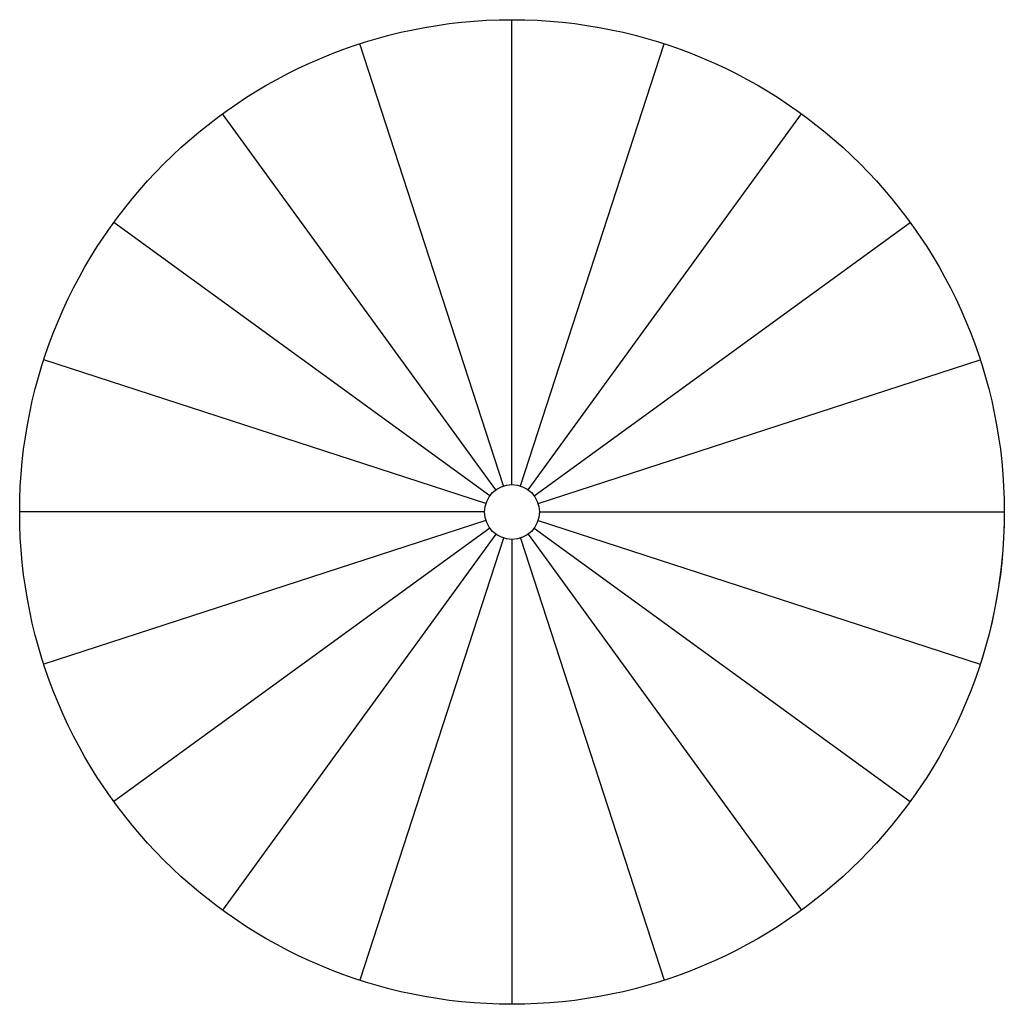
# Model space of a CAD drawing. Units: inches. Extents: x 32.9 to 104.9, y -12.7 to 59.3.
import ezdxf

# ---------------------------------------------------------------- set-up
doc = ezdxf.new("R2010")
doc.units = ezdxf.units.IN
doc.layers.add('A-FLOR-STRS', color=7, linetype='Continuous', lineweight=25)
doc.layers.add('M-CONS', color=9, linetype='Continuous', lineweight=13)

# ---------------------------------------------------------------- blocks, each defined once
blk = doc.blocks.new('*U1')
blk.add_line((-17, 0), (17, 0))
blk = doc.blocks.new('*U2')
at = {"layer": 'A-FLOR-STRS', "color": 0, "linetype": 'ByBlock', "lineweight": -2, "transparency": 16777216}
for p, rotation in [((68.939, 42.349), 89.99999999999989), ((63.068, 41.419), 107.9999999999998), ((74.81, 41.419), 71.9999999999999), ((57.771, 38.72), 125.9999999999998), ((80.107, 38.72), 53.99999999999995), ((53.568, 34.517), 143.9999999999997), ((84.31, 34.517), 35.99999999999994), ((50.869, 29.22), 161.9999999999997), ((87.009, 29.22), 17.99999999999997), ((49.939, 23.349), 180), ((50.869, 17.478), 197.9999999999997), ((87.009, 17.478), 341.9999999999995), ((53.568, 12.181), 215.9999999999997), ((57.771, 7.978), 233.9999999999996), ((80.107, 7.978), 305.9999999999996), ((84.31, 12.181), 323.9999999999995), ((63.068, 5.279), 251.9999999999996), ((68.939, 4.349), 269.9999999999995), ((74.81, 5.279), 287.9999999999996)]:
    blk.add_blockref('*U1', p, dxfattribs=dict(at, rotation=rotation))
blk.add_blockref('*U1', (87.939, 23.349), dxfattribs=at)

msp = doc.modelspace()

# ---------------------------------------------------------------- linework, layer by layer
at = {"layer": 'A-FLOR-STRS'}
for radius in [36, 2]:
    msp.add_circle((68.939, 23.349), radius, dxfattribs=at)
at = {"layer": 'M-CONS'}
msp.add_lwpolyline([(104.939, 23.349), (70.939, 23.349, -0.078702), (70.841, 22.731), (103.177, 12.224, 0.078702)], format="xyb", close=True, dxfattribs=at)

# ---------------------------------------------------------------- block references
at = {"layer": 'A-FLOR-STRS'}
msp.add_blockref('*U2', (0, 0), dxfattribs=at)

doc.saveas('drawing.dxf')
